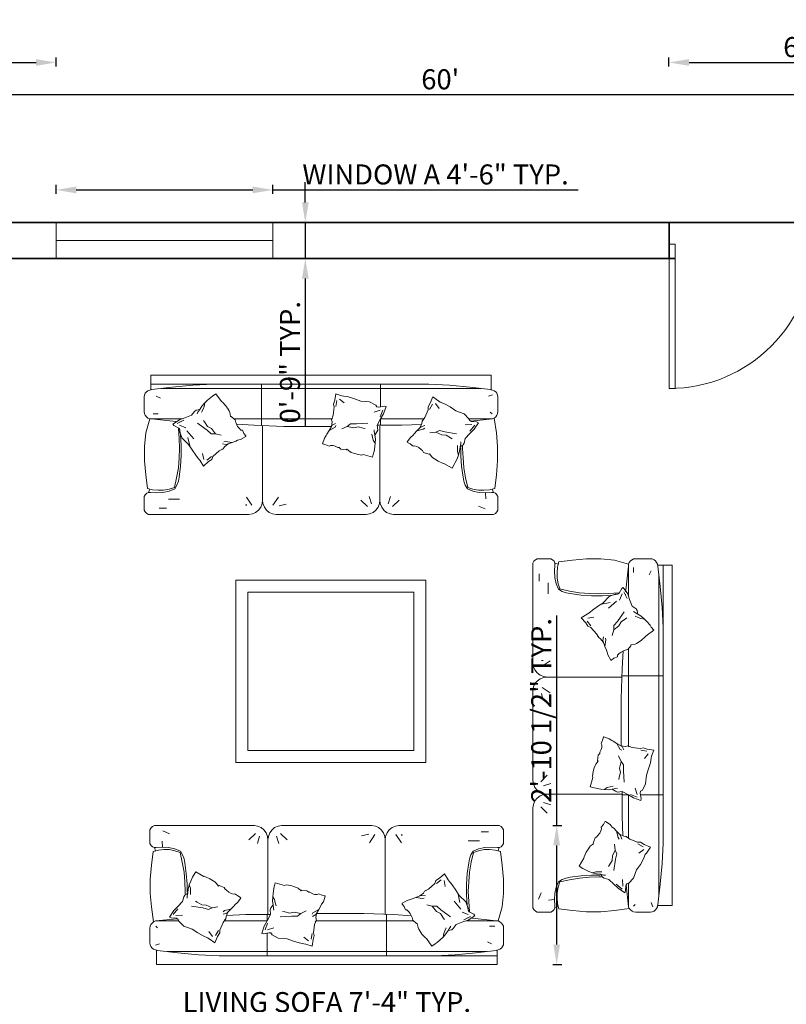
# Model space of a CAD drawing. Units: inches. Extents: x -100 to 766, y -562 to 63.
# Tile 9 of 11: x 257 to 448, y -182 to 63. Entities that reach past the tile are written whole.
import ezdxf

# ---------------------------------------------------------------- set-up
doc = ezdxf.new("R2010")
doc.units = ezdxf.units.IN
for name, color, linetype, lineweight in [('A-ANNO-DIMS', 2, 'Continuous', 18), ('A-DOOR', 3, 'Continuous', 18), ('A-GLAZ', 4, 'Continuous', 18), ('A-WALL', 7, 'Continuous', 35), ('furn', 8, 'Continuous', 13)]:
    doc.layers.add(name, color=color, linetype=linetype, lineweight=lineweight)
doc.styles.get("Standard").update_dxf_attribs({"font": 'arial.ttf'})
doc.dimstyles.new('ISO-25', dxfattribs={"dimtxt": 5, "dimasz": 5, "dimexe": 1.25, "dimexo": 0.625, "dimtad": 1, "dimlunit": 3, "dimtxsty": 'Standard', "dimcen": 2.5, "dimadec": 0, "dimazin": 0, "dimtfac": 1, "dimtmove": 0, "dimatfit": 3, "dimfxl": 1, "dimfxlon": 1, "dimarcsym": 0})

# ---------------------------------------------------------------- blocks, each defined once
blk = doc.blocks.new('*U2')
for p, q in [((0, 0), (0, -6)), ((40, 0), (40, -6))]:
    blk.add_line(p, q)
blk.add_lwpolyline([(0, 0), (0, 40), (1.75, 40), (1.75, 0)], close=True)
blk.add_arc((0, 0), 40, 0, 90)
blk = doc.blocks.new('sofa-43')
at = {"color": 0, "linetype": 'ByBlock'}
for p, q in [((-0.028, 0.939), (-0.038, 0.929)), ((-0.038, 0.929), (-0.028, 0.939)), ((-0.015, 0.947), (-0.028, 0.939)), ((-0.028, 0.939), (-0.015, 0.947)), ((-0.003, 0.947), (-0.015, 0.947)), ((-0.015, 0.947), (-0.003, 0.947)), ((0.665, 0.947), (-0.003, 0.947)), ((-0.003, 0.947), (0.665, 0.947)), ((0.687, 0.942), (0.665, 0.947)), ((0.687, 0.942), (0.665, 0.947)), ((0.712, 0.932), (0.687, 0.942)), ((0.712, 0.932), (0.687, 0.942)), ((0.827, 0.942), (0.802, 0.932)), ((0.802, 0.932), (0.827, 0.942)), ((0.85, 0.947), (0.827, 0.942)), ((0.827, 0.942), (0.85, 0.947)), ((1.462, 0.947), (0.85, 0.947)), ((0.85, 0.947), (1.462, 0.947)), ((1.487, 0.942), (1.462, 0.947)), ((1.487, 0.942), (1.462, 0.947)), ((1.509, 0.932), (1.487, 0.942)), ((1.509, 0.932), (1.487, 0.942)), ((1.624, 0.942), (1.602, 0.932)), ((1.602, 0.932), (1.624, 0.942)), ((1.647, 0.947), (1.624, 0.942)), ((1.624, 0.942), (1.647, 0.947)), ((2.317, 0.947), (1.647, 0.947)), ((1.647, 0.947), (2.317, 0.947)), ((2.329, 0.947), (2.317, 0.947)), ((2.329, 0.947), (2.317, 0.947)), ((2.342, 0.939), (2.329, 0.947)), ((2.342, 0.939), (2.329, 0.947)), ((2.352, 0.929), (2.342, 0.939)), ((2.352, 0.929), (2.342, 0.939)), ((-0.038, 0.929), (-0.045, 0.917)), ((-0.045, 0.917), (-0.038, 0.929)), ((-0.045, 0.917), (-0.045, 0.824)), ((-0.045, 0.917), (-0.045, 0.824)), ((0.042, 0.909), (0.087, 0.889)), ((0.672, 0.892), (0.627, 0.849)), ((0.7, 0.874), (0.685, 0.824)), ((0.73, 0.917), (0.712, 0.932)), ((0.73, 0.917), (0.712, 0.932)), ((0.745, 0.897), (0.73, 0.917)), ((0.745, 0.897), (0.73, 0.917)), ((0.755, 0.872), (0.745, 0.897)), ((0.755, 0.872), (0.745, 0.897)), ((0.757, 0.849), (0.755, 0.872)), ((0.757, 0.849), (0.755, 0.872)), ((0.76, 0.872), (0.757, 0.849)), ((0.757, 0.849), (0.76, 0.872)), ((0.77, 0.897), (0.76, 0.872)), ((0.76, 0.872), (0.77, 0.897)), ((0.785, 0.917), (0.77, 0.897)), ((0.77, 0.897), (0.785, 0.917)), ((0.802, 0.932), (0.785, 0.917)), ((0.785, 0.917), (0.802, 0.932)), ((0.815, 0.874), (0.83, 0.824)), ((0.842, 0.892), (0.887, 0.849)), ((1.442, 0.887), (1.394, 0.877)), ((1.484, 0.884), (1.447, 0.829)), ((1.527, 0.917), (1.509, 0.932)), ((1.527, 0.917), (1.509, 0.932)), ((1.542, 0.897), (1.527, 0.917)), ((1.542, 0.897), (1.527, 0.917)), ((1.552, 0.872), (1.542, 0.897)), ((1.552, 0.872), (1.542, 0.897)), ((1.554, 0.849), (1.552, 0.872)), ((1.554, 0.849), (1.552, 0.872)), ((1.557, 0.872), (1.554, 0.849)), ((1.554, 0.849), (1.557, 0.872)), ((1.567, 0.897), (1.557, 0.872)), ((1.557, 0.872), (1.567, 0.897)), ((1.582, 0.917), (1.567, 0.897)), ((1.567, 0.897), (1.582, 0.917)), ((1.602, 0.932), (1.582, 0.917)), ((1.582, 0.917), (1.602, 0.932)), ((1.627, 0.884), (1.664, 0.829)), ((1.667, 0.887), (1.667, 0.877)), ((2.257, 0.904), (2.207, 0.904)), ((2.359, 0.917), (2.352, 0.929)), ((2.359, 0.917), (2.352, 0.929)), ((2.359, 0.824), (2.359, 0.917)), ((2.359, 0.917), (2.359, 0.824)), ((-0.045, 0.824), (-0.038, 0.812)), ((-0.045, 0.824), (-0.038, 0.812)), ((-0.038, 0.812), (-0.028, 0.802)), ((-0.038, 0.812), (-0.028, 0.802)), ((0.04, 0.799), (0.037, 0.839)), ((0.757, 0.345), (0.757, 0.849)), ((1.554, 0.345), (1.554, 0.849)), ((2.194, 0.842), (2.119, 0.842)), ((2.342, 0.802), (2.352, 0.812)), ((2.352, 0.812), (2.342, 0.802)), ((2.352, 0.812), (2.359, 0.824)), ((2.359, 0.824), (2.352, 0.812)), ((-0.023, 0.769), (-0.035, 0.677)), ((-0.023, 0.769), (-0.035, 0.677)), ((-0.028, 0.802), (-0.015, 0.797)), ((-0.028, 0.802), (-0.015, 0.797)), ((0.012, 0.779), (-0.023, 0.769)), ((-0.0064, 0.7737), (-0.023, 0.769)), ((-0.015, 0.797), (-0.0064, 0.7737)), ((-0.015, 0.797), (-0.003, 0.797)), ((-0.0064, 0.7737), (-0.015, 0.797)), ((0.04, 0.799), (-0.003, 0.797)), ((0.05, 0.782), (0.012, 0.779)), ((0.082, 0.797), (0.04, 0.799)), ((0.087, 0.782), (0.05, 0.782)), ((0.125, 0.787), (0.082, 0.797)), ((0.125, 0.774), (0.087, 0.782)), ((0.162, 0.772), (0.125, 0.787)), ((0.16, 0.762), (0.125, 0.774)), ((0.175, 0.697), (0.16, 0.762)), ((0.177, 0.747), (0.162, 0.772)), ((0.187, 0.719), (0.177, 0.747)), ((2.127, 0.719), (2.137, 0.747)), ((2.137, 0.747), (2.152, 0.772)), ((2.139, 0.697), (2.154, 0.762)), ((2.152, 0.772), (2.189, 0.787)), ((2.154, 0.762), (2.189, 0.774)), ((2.189, 0.787), (2.232, 0.797)), ((2.189, 0.774), (2.227, 0.782)), ((2.227, 0.782), (2.264, 0.782)), ((2.232, 0.797), (2.274, 0.799)), ((2.264, 0.782), (2.302, 0.779)), ((2.274, 0.799), (2.317, 0.797)), ((2.302, 0.779), (2.337, 0.769)), ((2.329, 0.797), (2.317, 0.797)), ((2.3218, 0.7734), (2.329, 0.797)), ((2.3218, 0.7734), (2.329, 0.797)), ((2.337, 0.769), (2.3218, 0.7734)), ((2.329, 0.797), (2.342, 0.802)), ((2.342, 0.802), (2.329, 0.797)), ((2.349, 0.677), (2.337, 0.769)), ((2.337, 0.769), (2.349, 0.677)), ((-0.035, 0.677), (-0.043, 0.582)), ((-0.035, 0.677), (-0.043, 0.582)), ((0.187, 0.629), (0.175, 0.697)), ((0.192, 0.692), (0.187, 0.719)), ((0.202, 0.619), (0.192, 0.692)), ((2.112, 0.619), (2.122, 0.692)), ((2.122, 0.692), (2.127, 0.719)), ((2.127, 0.629), (2.139, 0.697)), ((2.357, 0.582), (2.349, 0.677)), ((2.349, 0.677), (2.357, 0.582)), ((0.192, 0.562), (0.187, 0.629)), ((0.207, 0.547), (0.202, 0.619)), ((0.252, 0.607), (0.245, 0.594)), ((0.267, 0.632), (0.252, 0.607)), ((0.322, 0.599), (0.267, 0.632)), ((1.957, 0.617), (1.922, 0.587)), ((1.982, 0.577), (1.957, 0.617)), ((2.107, 0.547), (2.112, 0.619)), ((2.122, 0.562), (2.127, 0.629)), ((-0.043, 0.582), (-0.043, 0.484)), ((-0.043, 0.582), (-0.043, 0.484)), ((0.195, 0.497), (0.192, 0.562)), ((0.207, 0.492), (0.207, 0.547)), ((0.222, 0.542), (0.215, 0.514)), ((0.232, 0.567), (0.222, 0.542)), ((0.222, 0.542), (0.23, 0.519)), ((0.245, 0.594), (0.232, 0.567)), ((0.332, 0.597), (0.322, 0.599)), ((0.362, 0.584), (0.332, 0.597)), ((0.385, 0.569), (0.362, 0.584)), ((0.397, 0.562), (0.385, 0.569)), ((0.405, 0.554), (0.397, 0.562)), ((0.42, 0.534), (0.405, 0.554)), ((0.425, 0.537), (0.42, 0.534)), ((0.46, 0.524), (0.425, 0.537)), ((0.807, 0.557), (0.8, 0.529)), ((0.87, 0.539), (0.807, 0.557)), ((0.88, 0.542), (0.87, 0.539)), ((0.912, 0.537), (0.88, 0.542)), ((0.937, 0.529), (0.912, 0.537)), ((1.892, 0.552), (1.849, 0.514)), ((1.899, 0.572), (1.892, 0.552)), ((1.922, 0.587), (1.899, 0.572)), ((1.934, 0.577), (1.902, 0.552)), ((1.954, 0.572), (1.962, 0.532)), ((1.989, 0.567), (1.982, 0.577)), ((2.009, 0.542), (1.989, 0.567)), ((2.034, 0.507), (2.009, 0.542)), ((2.107, 0.474), (2.107, 0.547)), ((2.119, 0.497), (2.122, 0.562)), ((2.357, 0.484), (2.357, 0.582)), ((2.357, 0.582), (2.357, 0.484)), ((-0.043, 0.484), (-0.035, 0.392)), ((-0.043, 0.484), (-0.035, 0.392)), ((0.192, 0.472), (0.185, 0.462)), ((0.212, 0.487), (0.192, 0.472)), ((0.195, 0.482), (0.195, 0.497)), ((0.207, 0.467), (0.212, 0.487)), ((0.215, 0.514), (0.212, 0.487)), ((0.23, 0.519), (0.23, 0.497)), ((0.23, 0.497), (0.23, 0.477)), ((0.467, 0.512), (0.46, 0.524)), ((0.475, 0.507), (0.467, 0.512)), ((0.492, 0.492), (0.475, 0.507)), ((0.507, 0.484), (0.492, 0.492)), ((0.522, 0.479), (0.507, 0.484)), ((0.532, 0.482), (0.522, 0.479)), ((0.552, 0.467), (0.532, 0.482)), ((0.792, 0.484), (0.79, 0.462)), ((0.797, 0.517), (0.792, 0.484)), ((0.8, 0.529), (0.797, 0.517)), ((0.952, 0.524), (0.937, 0.529)), ((0.962, 0.519), (0.952, 0.524)), ((0.982, 0.502), (0.962, 0.519)), ((0.987, 0.507), (0.982, 0.502)), ((1.022, 0.502), (0.987, 0.507)), ((1.035, 0.492), (1.022, 0.502)), ((1.042, 0.492), (1.035, 0.492)), ((1.062, 0.482), (1.042, 0.492)), ((1.074, 0.477), (1.062, 0.482)), ((1.092, 0.477), (1.074, 0.477)), ((1.102, 0.482), (1.092, 0.477)), ((1.124, 0.472), (1.102, 0.482)), ((1.144, 0.467), (1.124, 0.472)), ((1.814, 0.487), (1.789, 0.467)), ((1.789, 0.467), (1.802, 0.47)), ((1.802, 0.47), (1.827, 0.467)), ((1.822, 0.499), (1.814, 0.487)), ((1.849, 0.514), (1.822, 0.499)), ((1.827, 0.504), (1.832, 0.502)), ((2.057, 0.47), (2.034, 0.507)), ((2.062, 0.422), (2.049, 0.479)), ((2.102, 0.427), (2.057, 0.47)), ((2.112, 0.405), (2.107, 0.474)), ((2.122, 0.43), (2.119, 0.497)), ((2.349, 0.392), (2.357, 0.484)), ((2.357, 0.484), (2.349, 0.392)), ((0.177, 0.43), (0.145, 0.395)), ((0.185, 0.462), (0.177, 0.43)), ((0.207, 0.452), (0.207, 0.467)), ((0.277, 0.425), (0.265, 0.432)), ((0.307, 0.407), (0.277, 0.425)), ((0.337, 0.405), (0.307, 0.407)), ((0.377, 0.387), (0.337, 0.405)), ((0.525, 0.397), (0.532, 0.407)), ((0.532, 0.407), (0.55, 0.422)), ((0.55, 0.422), (0.572, 0.452)), ((0.57, 0.457), (0.552, 0.467)), ((0.572, 0.452), (0.57, 0.457)), ((0.792, 0.407), (0.777, 0.385)), ((0.79, 0.462), (0.787, 0.432)), ((0.787, 0.432), (0.792, 0.407)), ((0.79, 0.462), (0.802, 0.442)), ((0.795, 0.382), (0.792, 0.407)), ((0.802, 0.442), (0.807, 0.42)), ((0.807, 0.42), (0.812, 0.4)), ((1.117, 0.4), (1.122, 0.41)), ((1.122, 0.41), (1.134, 0.427)), ((1.134, 0.427), (1.147, 0.465)), ((1.147, 0.465), (1.144, 0.467)), ((1.704, 0.437), (1.669, 0.417)), ((1.669, 0.417), (1.669, 0.412)), ((1.669, 0.412), (1.682, 0.395)), ((1.724, 0.442), (1.704, 0.437)), ((1.737, 0.447), (1.724, 0.442)), ((1.762, 0.457), (1.737, 0.447)), ((1.789, 0.467), (1.762, 0.457)), ((1.762, 0.457), (1.807, 0.45)), ((1.807, 0.45), (1.819, 0.452)), ((1.874, 0.397), (1.837, 0.407)), ((2.069, 0.377), (2.022, 0.432)), ((2.119, 0.382), (2.102, 0.427)), ((2.117, 0.375), (2.112, 0.405)), ((2.127, 0.362), (2.122, 0.43)), ((-0.035, 0.392), (-0.02, 0.292)), ((-0.035, 0.392), (-0.02, 0.292)), ((0.117, 0.367), (0.087, 0.322)), ((0.112, 0.34), (0.145, 0.38)), ((0.145, 0.395), (0.117, 0.367)), ((0.132, 0.335), (0.177, 0.337)), ((0.237, 0.397), (0.315, 0.385)), ((0.315, 0.385), (0.352, 0.375)), ((0.352, 0.375), (0.377, 0.387)), ((0.377, 0.387), (0.417, 0.392)), ((0.462, 0.367), (0.452, 0.36)), ((0.477, 0.35), (0.452, 0.342)), ((0.505, 0.377), (0.462, 0.367)), ((0.472, 0.327), (0.485, 0.357)), ((0.607, 0.34), (0.475, 0.335)), ((0.485, 0.357), (0.477, 0.35)), ((0.485, 0.357), (0.505, 0.377)), ((0.505, 0.377), (0.525, 0.397)), ((0.775, 0.34), (0.607, 0.34)), ((0.775, 0.34), (0.752, 0.297)), ((0.752, 0.297), (0.752, 0.34)), ((0.777, 0.385), (0.772, 0.372)), ((0.772, 0.372), (0.775, 0.34)), ((0.797, 0.37), (0.795, 0.382)), ((0.872, 0.36), (0.857, 0.362)), ((0.905, 0.35), (0.872, 0.36)), ((0.935, 0.357), (0.905, 0.35)), ((0.98, 0.347), (0.935, 0.357)), ((0.957, 0.33), (0.98, 0.347)), ((0.98, 0.347), (1.017, 0.365)), ((1.062, 0.352), (1.057, 0.342)), ((1.082, 0.34), (1.059, 0.327)), ((1.102, 0.375), (1.062, 0.352)), ((1.087, 0.347), (1.082, 0.34)), ((1.082, 0.317), (1.087, 0.347)), ((1.087, 0.347), (1.102, 0.375)), ((1.409, 0.347), (1.087, 0.347)), ((1.102, 0.375), (1.117, 0.4)), ((1.612, 0.34), (1.409, 0.347)), ((1.562, 0.06), (1.562, 0.34)), ((1.732, 0.332), (1.612, 0.34)), ((1.682, 0.395), (1.692, 0.372)), ((1.692, 0.372), (1.702, 0.372)), ((1.702, 0.372), (1.714, 0.36)), ((1.714, 0.36), (1.724, 0.347)), ((1.724, 0.347), (1.734, 0.325)), ((1.874, 0.397), (1.902, 0.362)), ((1.904, 0.397), (1.874, 0.397)), ((1.902, 0.362), (1.929, 0.347)), ((1.932, 0.372), (1.904, 0.397)), ((1.929, 0.347), (1.949, 0.317)), ((1.997, 0.325), (1.932, 0.372)), ((2.119, 0.34), (2.077, 0.357)), ((2.117, 0.37), (2.119, 0.382)), ((2.124, 0.36), (2.117, 0.37)), ((2.157, 0.342), (2.124, 0.36)), ((2.129, 0.357), (2.127, 0.362)), ((2.164, 0.332), (2.157, 0.342)), ((2.322, 0.297), (2.349, 0.392)), ((2.349, 0.392), (2.322, 0.297)), ((-0.038, 0.272), (-0.043, 0.262)), ((-0.038, 0.272), (-0.043, 0.262)), ((-0.03, 0.282), (-0.038, 0.272)), ((-0.03, 0.282), (-0.038, 0.272)), ((-0.02, 0.292), (-0.03, 0.282)), ((-0.02, 0.292), (-0.03, 0.282)), ((-0.008, 0.297), (-0.02, 0.292)), ((0.14, 0.312), (-0.008, 0.297)), ((-0.008, 0.297), (0.15, 0.297)), ((0.005, 0.297), (-0.008, 0.297)), ((0.087, 0.322), (0.1, 0.317)), ((0.1, 0.317), (0.135, 0.315)), ((0.135, 0.315), (0.147, 0.307)), ((0.147, 0.307), (0.152, 0.295)), ((0.152, 0.295), (0.185, 0.262)), ((0.43, 0.235), (0.452, 0.287)), ((0.452, 0.287), (0.47, 0.312)), ((0.46, 0.297), (0.752, 0.297)), ((0.467, 0.307), (0.462, 0.307)), ((0.47, 0.312), (0.472, 0.327)), ((0.752, 0.297), (0.732, 0.262)), ((0.737, 0.237), (0.755, 0.282)), ((0.84, 0.325), (0.917, 0.33)), ((0.917, 0.33), (0.957, 0.33)), ((1.067, 0.217), (1.074, 0.272)), ((1.074, 0.272), (1.087, 0.302)), ((1.084, 0.297), (1.079, 0.292)), ((1.087, 0.302), (1.082, 0.317)), ((1.0855, 0.2985), (1.084, 0.297)), ((1.084, 0.297), (1.0848, 0.297)), ((1.084, 0.297), (1.562, 0.297)), ((1.0848, 0.297), (1.0855, 0.2985)), ((1.562, 0.297), (1.747, 0.297)), ((1.734, 0.325), (1.737, 0.32)), ((1.737, 0.32), (1.742, 0.302)), ((1.742, 0.302), (1.767, 0.28)), ((1.767, 0.28), (1.772, 0.28)), ((1.772, 0.28), (1.777, 0.252)), ((1.949, 0.317), (1.957, 0.307)), ((2.017, 0.245), (2.037, 0.272)), ((2.037, 0.272), (2.082, 0.29)), ((2.082, 0.29), (2.119, 0.302)), ((2.134, 0.327), (2.089, 0.305)), ((2.104, 0.297), (2.309, 0.297)), ((2.117, 0.317), (2.114, 0.317)), ((2.119, 0.302), (2.164, 0.332)), ((2.144, 0.315), (2.137, 0.317)), ((2.137, 0.315), (2.137, 0.317)), ((2.309, 0.297), (2.144, 0.315)), ((2.322, 0.297), (2.309, 0.297)), ((2.334, 0.292), (2.322, 0.297)), ((2.334, 0.292), (2.322, 0.297)), ((2.344, 0.282), (2.334, 0.292)), ((2.344, 0.282), (2.334, 0.292)), ((2.352, 0.272), (2.344, 0.282)), ((2.352, 0.272), (2.344, 0.282)), ((2.357, 0.262), (2.352, 0.272)), ((2.357, 0.262), (2.352, 0.272)), ((-0.043, 0.262), (-0.045, 0.247)), ((-0.043, 0.262), (-0.045, 0.247)), ((-0.045, 0.247), (-0.045, 0.147)), ((-0.045, 0.247), (-0.045, 0.147)), ((-0.005, 0.262), (0.007, 0.25)), ((0.185, 0.262), (0.242, 0.242)), ((0.242, 0.242), (0.28, 0.215)), ((0.28, 0.215), (0.317, 0.195)), ((0.38, 0.192), (0.355, 0.225)), ((0.4, 0.197), (0.42, 0.232)), ((0.415, 0.19), (0.43, 0.215)), ((0.43, 0.215), (0.43, 0.235)), ((0.732, 0.262), (0.715, 0.212)), ((0.715, 0.212), (0.727, 0.21)), ((0.727, 0.21), (0.765, 0.217)), ((0.752, 0.06), (0.752, 0.215)), ((0.755, 0.237), (0.797, 0.25)), ((0.765, 0.217), (0.777, 0.215)), ((0.777, 0.215), (0.785, 0.202)), ((0.785, 0.202), (0.827, 0.18)), ((1.05, 0.172), (1.057, 0.212)), ((1.072, 0.197), (1.067, 0.217)), ((1.777, 0.252), (1.782, 0.242)), ((1.782, 0.242), (1.789, 0.23)), ((1.789, 0.23), (1.804, 0.207)), ((1.804, 0.207), (1.827, 0.182)), ((1.947, 0.187), (1.952, 0.212)), ((1.947, 0.187), (1.967, 0.21)), ((1.952, 0.212), (1.959, 0.23)), ((1.959, 0.23), (1.969, 0.25)), ((1.967, 0.21), (1.982, 0.232)), ((1.994, 0.25), (1.982, 0.232)), ((1.982, 0.232), (2.007, 0.237)), ((1.999, 0.262), (1.994, 0.25)), ((2.007, 0.237), (2.017, 0.245)), ((2.299, 0.262), (2.264, 0.262)), ((2.359, 0.247), (2.357, 0.262)), ((2.359, 0.247), (2.357, 0.262)), ((2.359, 0.147), (2.359, 0.247)), ((2.359, 0.147), (2.359, 0.247)), ((-0.045, 0.147), (-0.043, 0.135)), ((-0.045, 0.147), (-0.043, 0.135)), ((-0.043, 0.135), (-0.038, 0.122)), ((-0.043, 0.135), (-0.038, 0.122)), ((-0.008, 0.132), (0.02, 0.142)), ((0.317, 0.195), (0.347, 0.182)), ((0.347, 0.182), (0.357, 0.175)), ((0.357, 0.175), (0.397, 0.147)), ((0.397, 0.147), (0.415, 0.19)), ((0.827, 0.18), (0.887, 0.175)), ((0.887, 0.175), (0.93, 0.16)), ((0.93, 0.16), (0.97, 0.147)), ((0.97, 0.147), (1.002, 0.142)), ((1.032, 0.162), (1, 0.187)), ((1.002, 0.142), (1.015, 0.14)), ((1.015, 0.14), (1.057, 0.125)), ((1.057, 0.125), (1.064, 0.17)), ((1.064, 0.17), (1.072, 0.197)), ((1.827, 0.182), (1.834, 0.177)), ((1.834, 0.177), (1.872, 0.125)), ((1.872, 0.125), (1.894, 0.142)), ((1.894, 0.142), (1.907, 0.15)), ((1.907, 0.15), (1.929, 0.17)), ((1.929, 0.17), (1.947, 0.187)), ((2.277, 0.142), (2.249, 0.155)), ((2.352, 0.122), (2.357, 0.135)), ((2.352, 0.122), (2.357, 0.135)), ((2.357, 0.135), (2.359, 0.147)), ((2.357, 0.135), (2.359, 0.147)), ((-0.038, 0.122), (-0.03, 0.112)), ((-0.038, 0.122), (-0.03, 0.112)), ((-0.03, 0.112), (-0.02, 0.105)), ((-0.03, 0.112), (-0.02, 0.105)), ((-0.02, 0.105), (-0.008, 0.1)), ((-0.02, 0.105), (-0.008, 0.1)), ((-0.008, 0.1), (0, 0.0982)), ((-0.008, 0.1), (0.005, 0.097)), ((0, 0.1), (0, 0)), ((0, 0.0982), (0, 0)), ((0.005, 0.097), (0.145, 0.08)), ((0.072, 0.09), (0.752, 0.09)), ((0.145, 0.08), (0.285, 0.067)), ((0.285, 0.067), (0.425, 0.06)), ((0.752, 0.09), (1.562, 0.09)), ((1.562, 0.09), (2.242, 0.09)), ((1.889, 0.06), (2.029, 0.067)), ((2.029, 0.067), (2.169, 0.08)), ((2.169, 0.08), (2.309, 0.097)), ((2.309, 0.097), (2.322, 0.1)), ((2.314, 0.0982), (2.322, 0.1)), ((2.314, 0.1), (2.314, 0)), ((2.314, 0), (2.314, 0.0982)), ((2.322, 0.1), (2.334, 0.105)), ((2.322, 0.1), (2.334, 0.105)), ((2.334, 0.105), (2.344, 0.112)), ((2.334, 0.105), (2.344, 0.112)), ((2.344, 0.112), (2.352, 0.122)), ((2.344, 0.112), (2.352, 0.122)), ((0, 0), (2.314, 0)), ((0, 0), (2.314, 0)), ((0.425, 0.06), (2.314, 0.06))]:
    blk.add_line(p, q, dxfattribs=at)
blk = doc.blocks.new('*D9')
at = {"layer": 'A-ANNO-DIMS', "color": 0, "lineweight": -2, "transparency": 16777216}
for p, q in [((1.39, 43.65), (1.39, 45.9)), ((6.39, 44.65), (716.39, 44.65)), ((721.39, 43.65), (721.39, 45.9))]:
    blk.add_line(p, q, dxfattribs=at)
at = {"layer": 'A-ANNO-DIMS', "color": 0, "transparency": 16777216}
for points in [[(6.39, 45.48), (6.39, 43.82), (1.39, 44.65)], [(716.39, 45.48), (716.39, 43.82), (721.39, 44.65)]]:
    blk.add_solid(points, dxfattribs=at)
at = {"layer": 'Defpoints', "color": 0, "transparency": 16777216}
for p in [(721.39, 44.65), (1.39, 12.79), (721.39, 12.79)]:
    blk.add_point(p, dxfattribs=at)
at = {"layer": 'A-ANNO-DIMS', "color": 0, "transparency": 16777216, "insert": (361.39, 47.83), "char_height": 5, "attachment_point": 5}
blk.add_mtext("60'", dxfattribs=at)
blk = doc.blocks.new('WIN-54IN')
blk.add_line((4.5, 54), (4.5, 0))
blk.add_lwpolyline([(0, 54), (9, 54), (9, 0), (0, 0)], close=True)
blk = doc.blocks.new('*D18')
at = {"layer": 'A-ANNO-DIMS', "color": 0, "lineweight": -2, "transparency": 16777216}
for p, q in [((265.66, 19.89), (265.66, 22.14)), ((319.66, 19.89), (319.66, 22.14)), ((270.66, 20.89), (314.66, 20.89)), ((319.66, 20.89), (395.78, 20.89))]:
    blk.add_line(p, q, dxfattribs=at)
at = {"layer": 'A-ANNO-DIMS', "color": 0, "transparency": 16777216}
for points in [[(270.66, 21.72), (270.66, 20.05), (265.66, 20.89)], [(314.66, 21.72), (314.66, 20.05), (319.66, 20.89)]]:
    blk.add_solid(points, dxfattribs=at)
at = {"layer": 'Defpoints', "color": 0, "transparency": 16777216}
for p in [(319.66, 20.89), (265.66, 12.79), (319.66, 12.79)]:
    blk.add_point(p, dxfattribs=at)
at = {"layer": 'A-ANNO-DIMS', "color": 0, "transparency": 16777216, "insert": (360.22, 24.1), "char_height": 5, "attachment_point": 5}
blk.add_mtext('WINDOW A 4\'-6" TYP.', dxfattribs=at)
blk = doc.blocks.new('*D19')
at = {"layer": 'A-ANNO-DIMS', "color": 0, "lineweight": -2, "transparency": 16777216}
for p, q in [((327.76, 17.79), (327.76, 22.79)), ((326.76, 12.79), (329.01, 12.79)), ((327.76, 12.79), (327.76, 3.79)), ((326.76, 3.79), (329.01, 3.79)), ((327.76, -1.21), (327.76, -37.94))]:
    blk.add_line(p, q, dxfattribs=at)
at = {"layer": 'A-ANNO-DIMS', "color": 0, "transparency": 16777216}
for points in [[(326.93, 17.79), (328.59, 17.79), (327.76, 12.79)], [(326.93, -1.21), (328.59, -1.21), (327.76, 3.79)]]:
    blk.add_solid(points, dxfattribs=at)
at = {"layer": 'Defpoints', "color": 0, "transparency": 16777216}
for p in [(319.66, 12.79), (319.66, 3.79), (327.76, 3.79)]:
    blk.add_point(p, dxfattribs=at)
at = {"layer": 'A-ANNO-DIMS', "color": 0, "transparency": 16777216, "insert": (324.58, -22.08), "char_height": 5, "attachment_point": 5, "rotation": 90}
blk.add_mtext('0\'-9" TYP.', dxfattribs=at)
blk = doc.blocks.new('*D26')
at = {"layer": 'A-ANNO-DIMS', "color": 0, "lineweight": -2, "transparency": 16777216}
for p, q in [((289.04, -184.53), (289.04, -186.78)), ((294.04, -185.53), (372.19, -185.53)), ((377.19, -184.53), (377.19, -186.78))]:
    blk.add_line(p, q, dxfattribs=at)
at = {"layer": 'A-ANNO-DIMS', "color": 0, "transparency": 16777216}
for points in [[(294.04, -184.7), (294.04, -186.37), (289.04, -185.53)], [(372.19, -184.7), (372.19, -186.37), (377.19, -185.53)]]:
    blk.add_solid(points, dxfattribs=at)
at = {"layer": 'Defpoints', "color": 0, "transparency": 16777216}
for p in [(289.04, -172.31), (377.19, -172.31), (377.19, -185.53)]:
    blk.add_point(p, dxfattribs=at)
at = {"layer": 'A-ANNO-DIMS', "color": 0, "transparency": 16777216, "insert": (333.12, -182.32), "char_height": 5, "attachment_point": 5}
blk.add_mtext('LIVING SOFA 7\'-4" TYP.', dxfattribs=at)
blk = doc.blocks.new('*D27')
at = {"layer": 'A-ANNO-DIMS', "color": 0, "lineweight": -2, "transparency": 16777216}
for p, q in [((390.41, -137.59), (390.41, -85.24)), ((389.41, -137.59), (391.66, -137.59)), ((390.41, -167.31), (390.41, -142.59)), ((389.41, -172.31), (391.66, -172.31))]:
    blk.add_line(p, q, dxfattribs=at)
at = {"layer": 'A-ANNO-DIMS', "color": 0, "transparency": 16777216}
for points in [[(389.57, -142.59), (391.24, -142.59), (390.41, -137.59)], [(389.57, -167.31), (391.24, -167.31), (390.41, -172.31)]]:
    blk.add_solid(points, dxfattribs=at)
at = {"layer": 'Defpoints', "color": 0, "transparency": 16777216}
for p in [(377.19, -137.59), (390.41, -137.59), (377.19, -172.31)]:
    blk.add_point(p, dxfattribs=at)
at = {"layer": 'A-ANNO-DIMS', "color": 0, "transparency": 16777216, "insert": (387.2, -108.92), "char_height": 5, "attachment_point": 5, "rotation": 90}
blk.add_mtext('2\'-10 1/2" TYP.', dxfattribs=at)
blk = doc.blocks.new('*D44')
at = {"layer": 'A-ANNO-DIMS', "color": 0, "lineweight": -2, "transparency": 16777216}
for p, q in [((418.39, 51.68), (418.39, 53.93)), ((423.39, 52.68), (485.39, 52.68)), ((490.39, 51.68), (490.39, 53.93))]:
    blk.add_line(p, q, dxfattribs=at)
at = {"layer": 'A-ANNO-DIMS', "color": 0, "transparency": 16777216}
for points in [[(423.39, 53.51), (423.39, 51.84), (418.39, 52.68)], [(485.39, 53.51), (485.39, 51.84), (490.39, 52.68)]]:
    blk.add_solid(points, dxfattribs=at)
at = {"layer": 'Defpoints', "color": 0, "transparency": 16777216}
for p in [(490.39, 52.68), (418.39, 12.79), (490.39, 12.79)]:
    blk.add_point(p, dxfattribs=at)
at = {"layer": 'A-ANNO-DIMS', "color": 0, "transparency": 16777216, "insert": (454.39, 55.86), "char_height": 5, "attachment_point": 5}
blk.add_mtext('6\'-0"', dxfattribs=at)
blk = doc.blocks.new('*D54')
at = {"layer": 'A-ANNO-DIMS', "color": 0, "lineweight": -2, "transparency": 16777216}
for p, q in [((-88.51, -62.62), (-90.76, -62.62)), ((-89.51, -67.62), (-89.51, -171.21)), ((-88.51, -176.21), (-90.76, -176.21))]:
    blk.add_line(p, q, dxfattribs=at)
at = {"layer": 'A-ANNO-DIMS', "color": 0, "transparency": 16777216}
for points in [[(-90.35, -67.62), (-88.68, -67.62), (-89.51, -62.62)], [(-90.35, -171.21), (-88.68, -171.21), (-89.51, -176.21)]]:
    blk.add_solid(points, dxfattribs=at)
at = {"layer": 'Defpoints', "color": 0, "transparency": 16777216}
for p in [(532.39, -62.62), (-89.51, -176.21), (532.39, -176.21)]:
    blk.add_point(p, dxfattribs=at)
at = {"layer": 'A-ANNO-DIMS', "color": 0, "transparency": 16777216, "insert": (-92.72, -119.41), "char_height": 5, "attachment_point": 5, "rotation": 90}
blk.add_mtext('9\'-5 1/2"', dxfattribs=at)
blk = doc.blocks.new('*D58')
at = {"layer": 'A-ANNO-DIMS', "color": 0, "lineweight": -2, "transparency": 16777216}
for p, q in [((189.91, 51.68), (189.91, 53.93)), ((194.91, 52.68), (260.66, 52.68)), ((265.66, 51.68), (265.66, 53.93))]:
    blk.add_line(p, q, dxfattribs=at)
at = {"layer": 'A-ANNO-DIMS', "color": 0, "transparency": 16777216}
for points in [[(194.91, 53.51), (194.91, 51.84), (189.91, 52.68)], [(260.66, 53.51), (260.66, 51.84), (265.66, 52.68)]]:
    blk.add_solid(points, dxfattribs=at)
at = {"layer": 'Defpoints', "color": 0, "transparency": 16777216}
for p in [(265.66, 52.68), (189.91, 12.79), (265.66, 12.79)]:
    blk.add_point(p, dxfattribs=at)
at = {"layer": 'A-ANNO-DIMS', "color": 0, "transparency": 16777216, "insert": (227.79, 55.89), "char_height": 5, "attachment_point": 5}
blk.add_mtext('6\'-3 1/2"', dxfattribs=at)
blk = doc.blocks.new('*D75')
at = {"layer": 'A-ANNO-DIMS', "color": 0, "lineweight": -2, "transparency": 16777216}
for p, q in [((-88.51, -37.21), (-90.76, -37.21)), ((-89.51, -42.21), (-89.51, -93.08)), ((-88.51, -98.08), (-90.76, -98.08))]:
    blk.add_line(p, q, dxfattribs=at)
at = {"layer": 'A-ANNO-DIMS', "color": 0, "transparency": 16777216}
for points in [[(-90.35, -42.21), (-88.68, -42.21), (-89.51, -37.21)], [(-90.35, -93.08), (-88.68, -93.08), (-89.51, -98.08)]]:
    blk.add_solid(points, dxfattribs=at)
at = {"layer": 'Defpoints', "color": 0, "transparency": 16777216}
for p in [(620.21, -37.21), (-89.51, -98.08), (620.21, -98.08)]:
    blk.add_point(p, dxfattribs=at)
at = {"layer": 'A-ANNO-DIMS', "color": 0, "transparency": 16777216, "insert": (-92.69, -67.65), "char_height": 5, "attachment_point": 5, "rotation": 90}
blk.add_mtext('5\'-1"', dxfattribs=at)
blk = doc.blocks.new('*D84')
at = {"layer": 'A-ANNO-DIMS', "color": 0, "lineweight": -2, "transparency": 16777216}
for p, q in [((-89.51, 8.79), (-89.51, 13.79)), ((-88.51, 3.79), (-90.76, 3.79)), ((-89.51, 3.79), (-89.51, -2.21)), ((-88.51, -2.21), (-90.76, -2.21)), ((-89.51, -7.21), (-89.51, -26.76))]:
    blk.add_line(p, q, dxfattribs=at)
at = {"layer": 'A-ANNO-DIMS', "color": 0, "transparency": 16777216}
for points in [[(-90.35, 8.79), (-88.68, 8.79), (-89.51, 3.79)], [(-90.35, -7.21), (-88.68, -7.21), (-89.51, -2.21)]]:
    blk.add_solid(points, dxfattribs=at)
at = {"layer": 'Defpoints', "color": 0, "transparency": 16777216}
for p in [(526.39, 3.79), (-89.51, -2.21), (526.39, -2.21)]:
    blk.add_point(p, dxfattribs=at)
at = {"layer": 'A-ANNO-DIMS', "color": 0, "transparency": 16777216, "insert": (-92.69, -19.49), "char_height": 5, "attachment_point": 5, "rotation": 90}
blk.add_mtext('0\'-6"', dxfattribs=at)
blk = doc.blocks.new('*D85')
at = {"layer": 'A-ANNO-DIMS', "color": 0, "lineweight": -2, "transparency": 16777216}
for p, q in [((761.28, -177.21), (761.28, -172.21)), ((760.28, -182.21), (762.53, -182.21)), ((761.28, -182.21), (761.28, -188.21)), ((760.28, -188.21), (762.53, -188.21)), ((761.28, -193.21), (761.28, -212.76))]:
    blk.add_line(p, q, dxfattribs=at)
at = {"layer": 'A-ANNO-DIMS', "color": 0, "transparency": 16777216}
for points in [[(760.45, -177.21), (762.11, -177.21), (761.28, -182.21)], [(760.45, -193.21), (762.11, -193.21), (761.28, -188.21)]]:
    blk.add_solid(points, dxfattribs=at)
at = {"layer": 'Defpoints', "color": 0, "transparency": 16777216}
for p in [(130.39, -182.21), (130.39, -188.21), (761.28, -188.21)]:
    blk.add_point(p, dxfattribs=at)
at = {"layer": 'A-ANNO-DIMS', "color": 0, "transparency": 16777216, "insert": (758.1, -205.49), "char_height": 5, "attachment_point": 5, "rotation": 90}
blk.add_mtext('0\'-6"', dxfattribs=at)
blk = doc.blocks.new('*D87')
at = {"layer": 'A-ANNO-DIMS', "color": 0, "lineweight": -2, "transparency": 16777216}
for p, q in [((310.41, -557.16), (310.41, -559.41)), ((357.79, -557.16), (357.79, -559.41)), ((315.41, -558.16), (352.79, -558.16))]:
    blk.add_line(p, q, dxfattribs=at)
at = {"layer": 'A-ANNO-DIMS', "color": 0, "transparency": 16777216}
for points in [[(315.41, -557.32), (315.41, -558.99), (310.41, -558.16)], [(352.79, -557.32), (352.79, -558.99), (357.79, -558.16)]]:
    blk.add_solid(points, dxfattribs=at)
at = {"layer": 'Defpoints', "color": 0, "transparency": 16777216}
for p in [(310.41, -121.91), (357.79, -121.91), (357.79, -558.16)]:
    blk.add_point(p, dxfattribs=at)
at = {"layer": 'A-ANNO-DIMS', "color": 0, "transparency": 16777216, "insert": (334.1, -554.94), "char_height": 5, "attachment_point": 5}
blk.add_mtext('3\'-11 1/2"', dxfattribs=at)
blk = doc.blocks.new('*D88')
at = {"layer": 'A-ANNO-DIMS', "color": 0, "lineweight": -2, "transparency": 16777216}
for p, q in [((-88.51, -76.41), (-90.76, -76.41)), ((-89.51, -81.41), (-89.51, -116.91)), ((-88.51, -121.91), (-90.76, -121.91))]:
    blk.add_line(p, q, dxfattribs=at)
at = {"layer": 'A-ANNO-DIMS', "color": 0, "transparency": 16777216}
for points in [[(-90.35, -81.41), (-88.68, -81.41), (-89.51, -76.41)], [(-90.35, -116.91), (-88.68, -116.91), (-89.51, -121.91)]]:
    blk.add_solid(points, dxfattribs=at)
at = {"layer": 'Defpoints', "color": 0, "transparency": 16777216}
for p in [(310.41, -76.41), (-89.51, -121.91), (310.41, -121.91)]:
    blk.add_point(p, dxfattribs=at)
at = {"layer": 'A-ANNO-DIMS', "color": 0, "transparency": 16777216, "insert": (-92.73, -99.16), "char_height": 5, "attachment_point": 5, "rotation": 90}
blk.add_mtext('3\'-9 1/2"', dxfattribs=at)

msp = doc.modelspace()

# ---------------------------------------------------------------- linework, layer by layer
at = {"layer": 'A-WALL'}
for p, q in [((418.394, 3.786), (418.394, 12.786)), ((229.388, 3.786), (271.388, 3.786)), ((271.388, 3.786), (419.97, 3.786))]:
    msp.add_line(p, q, dxfattribs=at)
msp.add_lwpolyline([(1.388, 12.786), (721.388, 12.786), (721.388, -467.214), (1.388, -467.214)], close=True, dxfattribs=at)
at = {"layer": 'furn'}
for points in [[(310.414, -76.409), (357.792, -76.409), (357.792, -121.911), (310.414, -121.911)], [(313.414, -79.409), (354.792, -79.409), (354.792, -118.911), (313.414, -118.911)]]:
    msp.add_lwpolyline(points, close=True, dxfattribs=at)

# ---------------------------------------------------------------- block references
at = {"layer": 'A-DOOR', "xscale": -0.900419896884199, "yscale": 0.900419896884199, "zscale": 0.900419896884199, "rotation": 180}
msp.add_blockref('*U2', (418.394, 7.383), dxfattribs=at)
at = {"layer": 'A-GLAZ', "rotation": 270.0000000000001}
msp.add_blockref('WIN-54IN', (265.66, 12.785), dxfattribs=at)
at = {"layer": 'furn', "xscale": 36.66436083614781, "yscale": 36.66436083614781, "zscale": 36.66436083614781}
for p, rotation in [((374.109, -25.35), 180), ((419.167, -157.572), 89.99999999999999)]:
    msp.add_blockref('sofa-43', p, dxfattribs=dict(at, rotation=rotation))
msp.add_blockref('sofa-43', (290.694, -172.311), dxfattribs=at)

# ---------------------------------------------------------------- dimensions: what is measured, and where the dimension line sits
at = {"layer": 'A-ANNO-DIMS'}
for base, p1, p2, override, picture, middle in [((265.66, 52.678), (189.914, 12.786), (265.66, 12.786), {"dimdec": 1, "dimlfac": 1, "dimrnd": 0, "dimzin": 1, "dimdsep": 46, "dimlunit": 4, "dimfrac": 2}, '*D58', (227.787, 55.89)), ((490.394, 52.678), (418.394, 12.786), (490.394, 12.786), {"dimdec": 1, "dimlfac": 1, "dimrnd": 0, "dimzin": 1, "dimdsep": 46, "dimlunit": 4, "dimfrac": 2}, '*D44', (454.394, 55.855)), ((721.388, 44.65), (1.388, 12.786), (721.388, 12.786), {"dimclrd": 0, "dimclre": 0, "dimclrt": 0}, '*D9', (361.388, 47.828)), ((357.792, -558.156), (310.414, -121.911), (357.792, -121.911), {"dimdec": 1, "dimlfac": 1, "dimrnd": 0, "dimzin": 1, "dimdsep": 46, "dimlunit": 4, "dimfrac": 2}, '*D87', (334.103, -554.944))]:
    dim = msp.add_linear_dim(base=base, p1=p1, p2=p2, dimstyle='ISO-25', override=override, dxfattribs=at)
    dim.commit()
    dim.dimension.update_dxf_attribs({"geometry": picture, "text_midpoint": middle})
for base, p1, p2, angle, text, picture, middle in [((319.66, 20.886), (265.66, 12.786), (319.66, 12.786), 0, 'WINDOW A <> TYP.', '*D18', (360.22, 24.098)), ((327.76, 3.786), (319.66, 12.786), (319.66, 3.786), 270, '<> TYP.', '*D19', (324.582, -22.078)), ((390.407, -137.589), (377.186, -172.311), (377.186, -137.589), 90, '<> TYP.', '*D27', (387.197, -108.915))]:
    dim = msp.add_linear_dim(base=base, p1=p1, p2=p2, angle=angle, text=text, dimstyle='ISO-25', override={"dimdec": 1, "dimlfac": 1, "dimrnd": 0, "dimzin": 1, "dimdsep": 46, "dimlunit": 4, "dimfrac": 2}, dxfattribs=at)
    dim.commit()
    dim.dimension.update_dxf_attribs({"geometry": picture, "text_midpoint": middle})
for base, p1, p2, picture, middle in [((-89.513, -2.214), (526.388, 3.786), (526.388, -2.214), '*D84', (-92.691, -19.485)), ((-89.513, -98.077), (620.215, -37.214), (620.215, -98.077), '*D75', (-92.691, -67.645)), ((-89.513, -176.214), (532.388, -62.615), (532.388, -176.214), '*D54', (-92.723, -119.415)), ((-89.513, -121.911), (310.414, -76.409), (310.414, -121.911), '*D88', (-92.725, -99.16)), ((761.28, -188.214), (130.388, -182.214), (130.388, -188.214), '*D85', (758.102, -205.485))]:
    dim = msp.add_linear_dim(base=base, p1=p1, p2=p2, angle=90, dimstyle='ISO-25', override={"dimdec": 1, "dimlfac": 1, "dimrnd": 0, "dimzin": 1, "dimdsep": 46, "dimlunit": 4, "dimfrac": 2}, dxfattribs=at)
    dim.commit()
    dim.dimension.update_dxf_attribs({"geometry": picture, "text_midpoint": middle})
dim = msp.add_linear_dim(base=(377.186, -185.532), p1=(289.045, -172.311), p2=(377.186, -172.311), text='LIVING SOFA <> TYP.', dimstyle='ISO-25', override={"dimdec": 1, "dimlfac": 1, "dimrnd": 0, "dimzin": 1, "dimdsep": 46, "dimlunit": 4, "dimfrac": 2}, dxfattribs=at)
dim.commit()
dim.dimension.update_dxf_attribs({"geometry": '*D26', "text_midpoint": (333.115, -182.32)})

doc.saveas('drawing.dxf')
